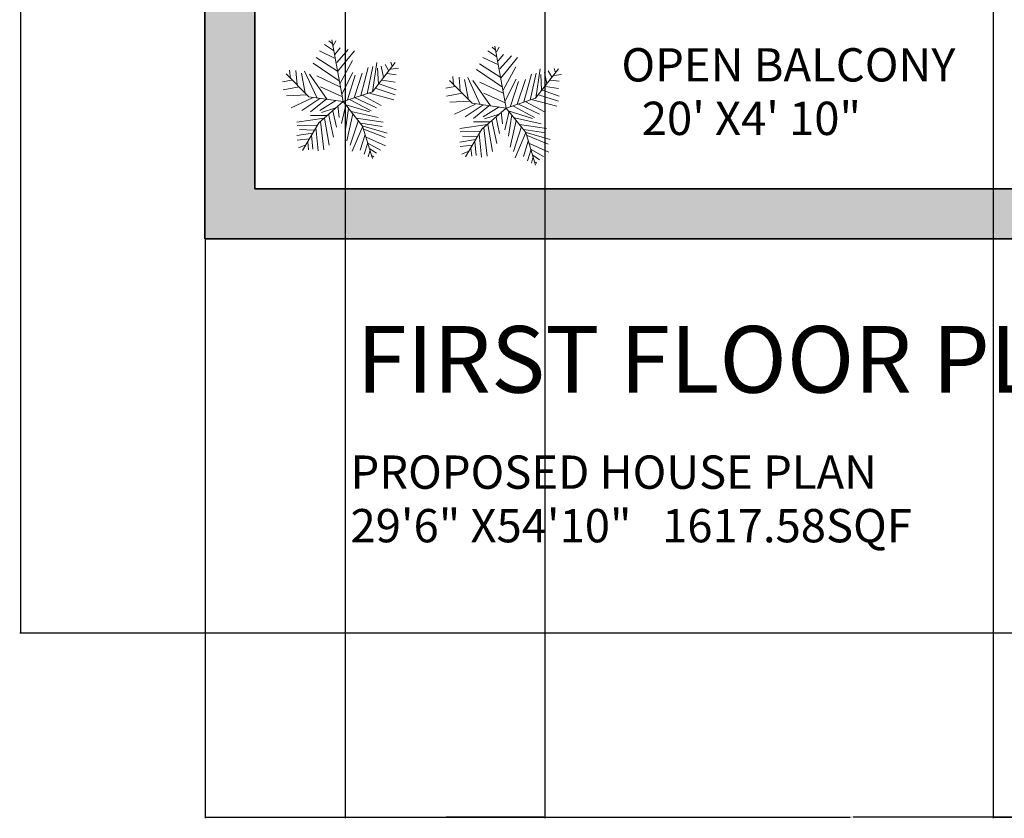
# Model space of a CAD drawing. Units: inches. Extents: x 2070 to 4408, y 1595 to 4269.
# Tile 1 of 20: x 2070 to 2247, y 1595 to 1739. Entities that reach past the tile are written whole.
import ezdxf

# ---------------------------------------------------------------- set-up
doc = ezdxf.new("R2010")
doc.units = ezdxf.units.IN
for name, color, linetype, lineweight in [('A-ANNO-DIMS', 2, 'Continuous', 18), ('A-ANNO-TITL', 7, 'Continuous', 25), ('A-AREA-IDEN', 7, 'Continuous', 18), ('A-WALL', 7, 'Continuous', 35), ('L-PLNT', 3, 'Continuous', 13)]:
    doc.layers.add(name, color=color, linetype=linetype, lineweight=lineweight)
doc.layers.add('A-WALL-PATT', color=18, linetype='Continuous', lineweight=13, true_color=0x000000)
doc.styles.get("Standard").update_dxf_attribs({"font": 'arial.ttf'})
doc.dimstyles.get("Standard").update_dxf_attribs({"dimtxt": 0.18, "dimasz": 0.18, "dimexe": 0.18, "dimexo": 0.0625, "dimgap": 0.09, "dimtad": 0, "dimtih": 1, "dimtoh": 1, "dimdec": 4, "dimzin": 0, "dimdsep": 46, "dimtxsty": 'Standard', "dimcen": 0.09, "dimadec": 0, "dimazin": 0, "dimtfac": 1, "dimtdec": 4, "dimtofl": 0, "dimtmove": 0, "dimatfit": 3, "dimfxl": 1, "dimtolj": 1, "dimtzin": 0, "dimarcsym": 0})

# ---------------------------------------------------------------- blocks, each defined once
blk = doc.blocks.new('Trees - Imperial')
for p, q in [((-10.186, 53.64), (-13.084, 55.962)), ((0, 0), (-10.5, 57)), ((-9.099, 51.782), (-6.563, 55.962)), ((-7.288, 39.707), (-21.778, 46.673)), ((-8.737, 47.138), (-17.069, 52.711)), ((-7.65, 43.423), (-2.578, 49.46)), ((-5.839, 35.992), (4.667, 48.067)), ((-5.114, 27.632), (10.463, 46.673)), ((-5.114, 28.097), (-24.676, 40.636)), ((-2.941, 16.486), (8.652, 37.85)), ((44.153, 36.456), (45.239, 32.741)), ((-48.585, 21.131), (-49.309, 29.026)), ((-43.513, 28.561), (-42.427, 15.558)), ((-35.544, 28.097), (-24.314, 3.947)), ((-3.665, 19.273), (-27.574, 35.527)), ((16.259, 5.805), (23.142, 31.348)), ((22.055, 7.198), (27.489, 32.277)), ((27, 9), (48, 36)), ((27.127, 9.056), (31.112, 35.992)), ((31.836, 30.883), (32.561, 16.486)), ((35.096, 32.741), (37.27, 22.524)), ((38.719, 34.134), (41.979, 28.561)), ((43.791, 29.954), (51.036, 30.883)), ((-47.498, 19.737), (-55.83, 18.344)), ((-31.5, 4.5), (-52.5, 25.5)), ((-38.442, 26.239), (-34.819, 7.663)), ((-14.533, 2.09), (-30.834, 25.31)), ((-24.314, 23.917), (-2.941, 13.7)), ((-1.129, 6.734), (9.014, 26.704)), ((3.942, 1.625), (11.187, 24.381)), ((10.101, 3.483), (17.708, 26.239)), ((36.183, 19.737), (48.137, 17.88)), ((40.53, 25.775), (48.862, 24.846)), ((-40.615, 13.7), (-55.105, 10.913)), ((-20.691, 13.7), (-1.129, 4.876)), ((29.662, 12.307), (48.137, 6.269)), ((33.285, 16.486), (48.862, 10.913)), ((-33.37, 6.269), (-52.207, 5.34)), ((-28.299, 3.483), (-47.86, -5.805)), ((-21.416, 3.018), (-38.079, -8.128)), ((0, 0), (-31.5, 4.5)), ((-15.982, 2.09), (-30.11, -9.521)), ((0, 0), (-22.5, -19.5)), ((-6.563, 1.161), (-21.416, -8.128)), ((0, 0), (27, 9)), ((0, 0), (18, -22.5)), ((6.478, 1.625), (26.04, -8.592)), ((11.187, 3.483), (30.749, -5.805)), ((18.07, 5.805), (35.096, -3.483)), ((24.229, 7.663), (46.688, 1.625)), ((-6.563, -5.805), (-19.967, -9.985)), ((-9.461, -8.592), (-6.201, -23.453)), ((-4.752, -3.483), (-3.665, -14.629)), ((2.493, -3.019), (-1.491, -20.202)), ((1.769, -2.555), (24.229, -9.521)), ((5.029, -6.27), (2.131, -25.775)), ((7.565, -9.056), (32.198, -14.629)), ((-17.431, -15.094), (-42.789, -18.809)), ((-15.257, -12.772), (-30.11, -12.772)), ((-17.069, -15.094), (-12.721, -40.172)), ((-13.446, -11.378), (-8.737, -32.741)), ((9.014, -11.378), (3.58, -35.992)), ((14.085, -16.951), (6.478, -40.172)), ((12.274, -15.094), (36.907, -18.809)), ((-24.314, -21.596), (-42.427, -22.06)), ((-26.849, -26.24), (-40.253, -25.775)), ((-22.5, -19.5), (-37.5, -45)), ((-25.038, -23.918), (-22.865, -45.281)), ((-20.691, -18.345), (-17.793, -44.352)), ((18.07, -22.524), (8.289, -45.745)), ((16.259, -19.738), (36.183, -22.989)), ((18, -22.5), (27, -52.5)), ((18.433, -22.524), (40.53, -29.026)), ((19.157, -25.311), (38.719, -33.206)), ((-28.299, -29.026), (-42.789, -31.348)), ((-30.834, -34.135), (-42.427, -35.528)), ((-29.023, -30.884), (-27.936, -43.887)), ((20.244, -30.419), (15.897, -44.816)), ((21.331, -32.741), (39.081, -40.636)), ((-34.457, -39.708), (-40.978, -42.494)), ((-32.646, -36.921), (-31.921, -44.352)), ((22.78, -37.85), (19.519, -48.532)), ((22.78, -38.314), (34.372, -44.816)), ((24.591, -43.423), (30.749, -47.603)), ((24.591, -45.745), (23.142, -50.854)), ((26.764, -49.925), (28.213, -50.854))]:
    blk.add_line(p, q)
blk = doc.blocks.new('*D24')
at = {"layer": 'A-ANNO-DIMS', "color": 0, "lineweight": -2, "transparency": 16777216}
for p, q in [((2103.13, 2291.4), (2069.84, 2291.4)), ((2070.02, 2291.22), (2070.02, 1960.08)), ((2070.02, 1628.58), (2070.02, 1959.72)), ((2336.13, 1628.4), (2069.84, 1628.4))]:
    blk.add_line(p, q, dxfattribs=at)
at = {"layer": 'A-ANNO-DIMS', "color": 0, "transparency": 16777216}
for points in [[(2069.99, 2291.22), (2070.05, 2291.22), (2070.02, 2291.4)], [(2069.99, 1628.58), (2070.05, 1628.58), (2070.02, 1628.4)]]:
    blk.add_solid(points, dxfattribs=at)
at = {"layer": 'Defpoints', "color": 0, "transparency": 16777216}
for p in [(2070.02, 2291.4), (2103.2, 2291.4), (2336.2, 1628.4)]:
    blk.add_point(p, dxfattribs=at)
at = {"layer": 'A-ANNO-DIMS', "color": 0, "transparency": 16777216, "insert": (2070.02, 1959.9), "char_height": 0.18, "attachment_point": 5}
blk.add_mtext('\\A1;663', dxfattribs=at)
blk = doc.blocks.new('*D25')
at = {"layer": 'A-ANNO-DIMS', "color": 0, "lineweight": -2, "transparency": 16777216}
for p, q in [((2103.2, 1699.34), (2103.2, 1595.04)), ((2336.2, 1699.34), (2336.2, 1595.04)), ((2103.38, 1595.22), (2219.41, 1595.22)), ((2336.02, 1595.22), (2219.99, 1595.22))]:
    blk.add_line(p, q, dxfattribs=at)
at = {"layer": 'A-ANNO-DIMS', "color": 0, "transparency": 16777216}
for points in [[(2103.38, 1595.25), (2103.38, 1595.19), (2103.2, 1595.22)], [(2336.02, 1595.25), (2336.02, 1595.19), (2336.2, 1595.22)]]:
    blk.add_solid(points, dxfattribs=at)
at = {"layer": 'Defpoints', "color": 0, "transparency": 16777216}
for p in [(2103.2, 1699.4), (2336.2, 1699.4), (2336.2, 1595.22)]:
    blk.add_point(p, dxfattribs=at)
at = {"layer": 'A-ANNO-DIMS', "color": 0, "transparency": 16777216, "insert": (2219.7, 1595.22), "char_height": 0.18, "attachment_point": 5}
blk.add_mtext('\\A1;233', dxfattribs=at)
blk = doc.blocks.new('*D29')
at = {"layer": 'A-ANNO-DIMS', "color": 0, "lineweight": -2, "transparency": 16777216}
for p, q in [((2128.44, 2150.34), (2128.44, 1595.04)), ((2164.44, 2150.34), (2164.44, 1595.04)), ((2128.62, 1595.22), (2146.22, 1595.22)), ((2164.26, 1595.22), (2146.65, 1595.22))]:
    blk.add_line(p, q, dxfattribs=at)
at = {"layer": 'A-ANNO-DIMS', "color": 0, "transparency": 16777216}
for points in [[(2128.62, 1595.25), (2128.62, 1595.19), (2128.44, 1595.22)], [(2164.26, 1595.25), (2164.26, 1595.19), (2164.44, 1595.22)]]:
    blk.add_solid(points, dxfattribs=at)
at = {"layer": 'Defpoints', "color": 0, "transparency": 16777216}
for p in [(2128.44, 2150.4), (2164.44, 2150.4), (2164.44, 1595.22)]:
    blk.add_point(p, dxfattribs=at)
at = {"layer": 'A-ANNO-DIMS', "color": 0, "transparency": 16777216, "insert": (2146.44, 1595.22), "char_height": 0.18, "attachment_point": 5}
blk.add_mtext('\\A1;36', dxfattribs=at)
blk = doc.blocks.new('*D32')
at = {"layer": 'A-ANNO-DIMS', "color": 0, "lineweight": -2, "transparency": 16777216}
for p, q in [((2245.2, 2230.58), (2245.2, 1595.04)), ((2340.2, 2230.58), (2340.2, 1595.04)), ((2245.38, 1595.22), (2292.48, 1595.22)), ((2340.02, 1595.22), (2292.92, 1595.22))]:
    blk.add_line(p, q, dxfattribs=at)
at = {"layer": 'A-ANNO-DIMS', "color": 0, "transparency": 16777216}
for points in [[(2245.38, 1595.25), (2245.38, 1595.19), (2245.2, 1595.22)], [(2340.02, 1595.25), (2340.02, 1595.19), (2340.2, 1595.22)]]:
    blk.add_solid(points, dxfattribs=at)
at = {"layer": 'Defpoints', "color": 0, "transparency": 16777216}
for p in [(2245.2, 2230.65), (2340.2, 2230.65), (2340.2, 1595.22)]:
    blk.add_point(p, dxfattribs=at)
at = {"layer": 'A-ANNO-DIMS', "color": 0, "transparency": 16777216, "insert": (2292.7, 1595.22), "char_height": 0.18, "attachment_point": 5}
blk.add_mtext('\\A1;95', dxfattribs=at)

msp = doc.modelspace()

# ---------------------------------------------------------------- hatches: boundary and pattern name
at = {"layer": 'A-WALL-PATT'}
h = msp.add_hatch(color=256, dxfattribs=at)
h.dxf.hatch_style = 1
h.paths.add_polyline_path([(2346.196, 2218.3995), (2346.196, 2282.3995), (2340.196, 2282.3995), (2340.196, 2212.3995), (2345.5866, 2212.3995), (2346.196, 2212.3995)], flags=0)
h.paths.add_polyline_path([(2245.196, 2282.3995), (2239.196, 2282.3995), (2239.196, 2186.3995), (2244.5866, 2186.3995), (2245.196, 2186.3995)], flags=0)
h.paths.add_polyline_path([(2340.196, 2230.6455), (2245.196, 2230.6455), (2245.196, 2224.6455), (2340.196, 2224.6455)], flags=0)
h.paths.add_polyline_path([(2245.196, 2150.3995), (2239.196, 2150.3995), (2164.4362, 2150.3995), (2164.4362, 2144.3995), (2239.196, 2144.3995), (2239.196, 2086.3995), (2239.196, 2067.2711), (2244.5866, 2067.2711), (2245.196, 2067.2711), (2245.196, 2144.3995)], flags=0)
h.paths.add_polyline_path([(2346.196, 2176.3995), (2340.196, 2176.3995), (2340.196, 2086.3995), (2346.196, 2086.3995), (2346.196, 2125.318)], flags=0)
h.paths.add_polyline_path([(2446.196, 2086.3995), (2346.196, 2086.3995), (2340.196, 2086.3995), (2340.196, 2080.3995), (2446.196, 2080.3995)], flags=0)
h.paths.add_polyline_path([(2455.196, 2291.3995), (2103.196, 2291.3995), (2103.196, 1699.3995), (2336.196, 1699.3995), (2336.196, 1628.3995), (2345.196, 1628.3995), (2446.196, 1628.3995), (2454.8846, 1628.3995), (2454.8846, 1699.3995)])
h.paths.add_polyline_path([(2446.196, 2282.3995), (2446.196, 2218.3995), (2446.196, 2212.3995), (2446.196, 2086.3995), (2446.196, 2080.3995), (2446.196, 1708.3995), (2446.196, 1637.3995), (2345.196, 1637.3995), (2345.196, 1699.3995), (2345.196, 1708.3995), (2336.196, 1708.3995), (2112.196, 1708.3995), (2112.196, 2282.3995), (2239.196, 2282.3995), (2245.196, 2282.3995), (2356.196, 2282.3995)], flags=16)
h.paths.add_polyline_path([(2245.196, 2150.3995), (2245.196, 2144.3995), (2245.196, 2067.2711), (2244.5866, 2067.2711), (2239.196, 2067.2711), (2239.196, 2065.6988), (2203.2929, 2065.6988, 0.40145271), (2239.196, 2031.3337), (2244.5866, 2031.3337), (2245.196, 2031.2711), (2245.196, 1924.1525), (2239.196, 1924.1525), (2239.196, 1922.5803), (2203.2929, 1922.5803, 0.40145271), (2239.196, 1888.2151), (2244.5866, 1888.2151), (2245.196, 1888.1525), (2245.196, 1748.3995), (2339.196, 1748.4621, -0.40145271), (2303.2929, 1782.8272), (2303.2585, 1782.8272), (2303.2585, 1784.3995), (2339.196, 1784.3995), (2339.196, 1877.2067), (2291.196, 1877.2067), (2291.196, 1883.2067), (2291.196, 1946.3995), (2291.196, 1952.3995), (2291.196, 2086.3995), (2297.196, 2086.3995), (2302.196, 2086.3995), (2302.196, 2081.0259), (2303.7633, 2081.0259), (2303.7633, 2080.3995), (2338.0148, 2080.3995, 0.00437129), (2338.0203, 2081.0259), (2338.0203, 2086.3995), (2340.196, 2086.3995), (2340.196, 2176.4621), (2345.5866, 2176.4621, 0.40145271), (2381.4896, 2210.8272), (2345.5866, 2210.8272), (2345.5866, 2212.3995), (2340.196, 2212.3995), (2340.196, 2224.6455), (2245.196, 2224.6455), (2245.196, 2186.3995), (2244.5866, 2186.3995), (2239.196, 2186.3995), (2239.196, 2184.8272), (2203.2929, 2184.8272, 0.40145271), (2239.196, 2150.4621), (2244.5866, 2150.4621)], flags=0)
h.paths.add_polyline_path([(2346.196, 2282.3995), (2346.196, 2218.3995), (2377.1813, 2218.3995), (2377.1813, 2212.3995), (2346.196, 2212.3995), (2345.5866, 2212.3995), (2340.196, 2212.3995), (2340.196, 2224.6455), (2245.196, 2224.6455), (2245.196, 2230.6455), (2245.196, 2282.3995), (2292.696, 2256.5225), (2340.196, 2282.3995)], flags=0)
h.paths.add_polyline_path([(2346.196, 2086.3995), (2340.196, 2086.3995), (2340.196, 2080.3995), (2446.196, 2080.3995), (2431.196, 2016.3995), (2446.196, 1952.3995), (2412.196, 1952.3995), (2412.196, 2080.3995), (2340.196, 2080.3995), (2340.196, 2086.3995), (2340.196, 2176.3995), (2346.196, 2176.3995), (2346.196, 2125.318)], flags=0)
h.paths.add_polyline_path([(2186.508, 2270.0471, -0.03755288), (2186.9712, 2269.8581), (2186.9164, 2270.112, -0.02759121)], flags=0)
h.paths.add_polyline_path([(2183.955, 2273.7766, 1), (2188.2945, 2273.7766, 1)], flags=0)
h.paths.add_polyline_path([(2142.5261, 2274.6158, -0.03707541), (2142.5672, 2275.1696), (2142.5672, 2276.826), (2119.8759, 2276.826), (2119.8759, 2263.0962), (2140.4332, 2263.0962), (2142.5672, 2263.0962), (2142.5672, 2274.0621, -0.03707541)], flags=0)
h.paths.add_polyline_path([(2209.8974, 2263.0962), (2209.8974, 2262.2079), (2190.8042, 2262.2079), (2190.8042, 2263.0962)], flags=0)
h.paths.add_polyline_path([(2210.6382, 2276.1833), (2210.6382, 2263.9844), (2190.2185, 2263.9844), (2190.2185, 2276.1833)], flags=0)
h.paths.add_polyline_path([(2188.4362, 2273.7766, -1), (2183.8133, 2273.7766, -1)], flags=0)
h.paths.add_polyline_path([(2245.196, 2150.3995), (2245.196, 2144.3995), (2245.196, 2067.2711), (2239.196, 2067.2711), (2239.196, 2080.3995), (2172.196, 2080.3995), (2172.196, 2000.3995), (2239.196, 2000.3995), (2239.196, 1940.3995), (2159.0187, 1940.3995), (2123.0187, 1940.3995), (2112.196, 1940.3995), (2112.196, 1946.3995), (2123.0187, 1946.3995), (2123.0187, 1982.2238), (2124.586, 1982.2238), (2124.586, 1982.1895, -0.40145271), (2158.8429, 1946.3995), (2159.0187, 1946.3995), (2239.196, 1946.3995), (2239.196, 1994.3995), (2112.196, 1994.3995), (2112.196, 2000.3995), (2139.196, 2040.3995), (2112.196, 2080.3995), (2112.196, 2086.3995), (2239.196, 2086.3995), (2239.196, 2144.3995), (2209.5809, 2144.3995), (2209.5809, 2136.3995), (2203.0809, 2136.3995), (2205.0809, 2130.3996, -0.70257121), (2199.081, 2116.3995, -0.70256205), (2193.0809, 2130.3994), (2195.0809, 2136.3995), (2192.0809, 2136.3995), (2192.0809, 2134.8995), (2189.0809, 2134.8995), (2189.0809, 2135.8995), (2191.0809, 2135.8995), (2191.0809, 2136.3995), (2188.5809, 2136.3995), (2188.5809, 2144.3995), (2164.2481, 2144.3995, -0.39385849), (2130.0035, 2109.5491), (2130.0035, 2109.5147), (2128.4362, 2109.5147), (2128.4362, 2144.3995), (2112.196, 2144.3995), (2112.196, 2150.3995), (2128.4362, 2150.3995), (2128.4362, 2150.7127), (2164.4362, 2150.7127), (2164.4362, 2150.3995), (2239.196, 2150.3995)], flags=0)
h.paths.add_polyline_path([(2188.2075, 2266.8735), (2188.2075, 2211.8632, -0.41421356), (2185.4833, 2209.1391), (2146.7995, 2209.1391, -0.41421356), (2144.0754, 2211.8632), (2144.0754, 2266.8735, -0.41421356), (2146.7995, 2269.5976), (2185.4833, 2269.5976, -0.41421356)], flags=0)
h.paths.add_polyline_path([(2185.0844, 2273.7766, -1), (2187.1651, 2273.7766, -1)], flags=0)
h.paths.add_polyline_path([(2182.0486, 2259.2932), (2168.0953, 2259.2932), (2168.0953, 2260.8424), (2163.7261, 2260.8424), (2163.7261, 2259.2932), (2149.7727, 2259.2932), (2149.7727, 2266.3352), (2163.7261, 2266.3352), (2163.7261, 2261.9839), (2168.0953, 2261.9839), (2168.0953, 2266.3352), (2182.0486, 2266.3352)], flags=0)
h.paths.add_polyline_path([(2148.2585, 2250.2051), (2153.0615, 2241.8861, 0.39807048)], flags=0)
h.paths.add_polyline_path([(2162.7572, 2247.2885), (2153.1461, 2241.7396), (2148.1083, 2250.4653), (2157.7194, 2256.0142)], flags=0)
h.paths.add_polyline_path([(2162.6726, 2247.4351, -0.39286196), (2157.8415, 2255.6313), (2157.6431, 2255.6313), (2157.8696, 2255.7541)], flags=0)
h.paths.add_polyline_path([(2164.2604, 2145.339), (2164.4362, 2144.3995), (2164.4362, 2150.3995), (2164.2604, 2150.7127)], flags=0)
h.paths.add_polyline_path([(2208.5809, 2142.6495), (2208.5809, 2138.3995, -0.41421356), (2207.8309, 2137.3995), (2190.5809, 2137.3995, -0.41421356), (2189.5809, 2138.1495), (2189.5809, 2142.3995, -0.41421356), (2190.3309, 2143.3995), (2207.5809, 2143.3995, -0.41421356)], flags=0)
h.paths.add_polyline_path([(2147.957, 2229.9119), (2154.7494, 2223.1195, 0.39807048)], flags=0)
h.paths.add_polyline_path([(2162.7165, 2230.8473), (2154.8691, 2222.9998), (2147.7446, 2230.1244), (2155.592, 2237.9718)], flags=0)
h.paths.add_polyline_path([(2162.5969, 2230.9669, -0.39807048), (2155.8044, 2237.7594)], flags=0)
h.paths.add_polyline_path([(2391.8776, 2049.9192), (2408.5766, 2049.9192), (2408.5766, 2033.2202), (2408.5766, 1983.123), (2408.5766, 1966.4239), (2391.8776, 1966.4239), (2391.8776, 1983.123), (2341.7804, 1983.123), (2341.7804, 2033.2202), (2391.8776, 2033.2202)], flags=0)
h.paths.add_polyline_path([(2144.1055, 2274.6158, 1), (2148.445, 2274.6158, 1)], flags=0)
h.paths.add_polyline_path([(2148.5867, 2274.6158, -1), (2143.9638, 2274.6158, -1)], flags=0)
h.paths.add_polyline_path([(2145.2349, 2274.6158, -1), (2147.3156, 2274.6158, -1)], flags=0)
edge = h.paths.add_edge_path(flags=0)
edge.add_ellipse((2400.5951, 2040.9436), major_axis=(-4.5109, 0), ratio=0.97544784, start_angle=180, end_angle=270, ccw=False)
edge.add_ellipse((2400.5951, 2040.9436), major_axis=(-4.5109, 0), ratio=0.97544784, start_angle=90, end_angle=180, ccw=False)
edge.add_ellipse((2400.5951, 2040.9436), major_axis=(-4.5109, 0), ratio=0.97544784, start_angle=0, end_angle=90, ccw=False)
edge.add_ellipse((2400.5951, 2040.9436), major_axis=(-4.5109, 0), ratio=0.97544784, start_angle=270, end_angle=360, ccw=False)
h.paths.add_polyline_path([(2199.0809, 2117.3995, -0.73452973), (2195.0809, 2130.3995), (2203.081, 2130.3995, -0.73453329)], flags=0)
h.paths.add_polyline_path([(2141.9147, 2276.0353), (2141.9147, 2263.9844), (2120.4685, 2263.9844), (2120.4685, 2276.0353)], flags=0)
h.paths.add_polyline_path([(2138.4481, 2273.4072), (2138.4481, 2266.7226), (2133.2801, 2266.7226), (2133.2801, 2273.4072)], flags=0)
h.paths.add_polyline_path([(2137.9691, 2272.9175), (2137.9691, 2272.204), (2135.4229, 2272.204), (2135.4229, 2271.6329), (2135.3221, 2270.1051), (2135.3221, 2269.0265), (2135.4229, 2268.6811), (2135.4229, 2267.2011), (2133.7212, 2267.2011), (2133.7212, 2268.6811), (2133.7983, 2269.9587), (2133.7983, 2271.2758), (2133.7212, 2271.6329), (2133.7212, 2273.0065), (2135.717, 2273.0065), (2135.717, 2272.9175)], flags=0)
h.paths.add_polyline_path([(2137.9215, 2271.8264), (2137.9215, 2271.3786), (2137.5182, 2271.3786), (2136.9355, 2271.3786), (2136.3529, 2271.3786), (2135.7703, 2271.3786), (2135.7703, 2271.8264), (2136.1736, 2271.8264), (2136.7562, 2271.8264), (2137.3389, 2271.8264)], flags=0)
h.paths.add_polyline_path([(2137.9215, 2271.692), (2137.5182, 2271.692), (2136.9355, 2271.513), (2137.3389, 2271.513)], flags=0)
h.paths.add_polyline_path([(2136.3529, 2271.692), (2135.7703, 2271.513), (2136.1736, 2271.513), (2136.7562, 2271.692)], flags=0)
h.paths.add_polyline_path([(2137.9215, 2271.513), (2137.5182, 2271.513), (2136.7562, 2271.747), (2136.7562, 2271.692), (2137.3389, 2271.692)], flags=0)
h.paths.add_polyline_path([(2137.8207, 2270.4664), (2137.8207, 2270.0971), (2137.8207, 2269.627), (2137.8207, 2269.1569), (2137.8207, 2268.6868), (2137.3837, 2268.6868), (2136.6442, 2268.6868), (2135.9271, 2268.6868), (2135.9271, 2269.0562), (2135.9271, 2269.5263), (2135.9271, 2269.9963), (2135.9271, 2270.4664), (2136.3641, 2270.4664), (2137.0812, 2270.4664)], flags=0)
h.paths.add_polyline_path([(2137.3837, 2269.627), (2137.8207, 2269.627), (2137.8207, 2269.5263), (2137.3837, 2269.5263), (2137.3837, 2269.1569), (2137.8207, 2269.1569), (2137.3837, 2269.0562), (2137.3837, 2268.6868), (2137.0812, 2268.6868), (2137.0812, 2269.0562), (2136.6442, 2269.0562), (2136.6442, 2268.6868), (2136.3641, 2268.6868), (2136.3641, 2269.0562), (2135.9271, 2269.0562), (2135.9271, 2269.1569), (2136.3641, 2269.1569), (2136.3641, 2269.5263), (2135.9271, 2269.5263), (2135.9271, 2269.627), (2136.3641, 2269.627), (2136.3641, 2269.9963), (2135.9271, 2269.9963), (2136.3641, 2270.0971), (2136.3641, 2270.4664), (2136.6442, 2270.4664), (2136.6442, 2270.0971), (2137.0812, 2270.0971), (2137.0812, 2270.4664), (2137.3837, 2270.4664), (2137.3837, 2270.0971), (2137.8207, 2270.0971), (2137.3837, 2269.9963)], flags=0)
h.paths.add_polyline_path([(2137.5182, 2271.8264), (2137.5182, 2271.692), (2137.3389, 2271.3786), (2137.3389, 2271.513)], flags=0)
h.paths.add_polyline_path([(2137.8179, 2267.8138), (2137.8179, 2267.6879), (2137.1876, 2267.6879), (2136.4733, 2267.6879), (2135.759, 2267.6879), (2135.759, 2267.8138), (2136.3893, 2267.8138), (2137.1036, 2267.8138)], flags=0)
h.paths.add_polyline_path([(2137.0812, 2269.9963), (2137.0812, 2269.627), (2137.0812, 2269.1569), (2136.6442, 2269.1569), (2136.6442, 2269.5263), (2136.6442, 2269.9963)], flags=0)
h.paths.add_polyline_path([(2136.3529, 2271.8264), (2136.3529, 2271.692), (2136.1736, 2271.3786), (2136.1736, 2271.513)], flags=0)
h.paths.add_polyline_path([(2136.4733, 2267.8138), (2136.4733, 2267.6879), (2136.3893, 2267.6879), (2136.3893, 2267.8138)], flags=0)
h.paths.add_polyline_path([(2407.9087, 2032.5522), (2407.9087, 1983.7909), (2359.81, 1983.7909, -0.00912788), (2359.0575, 1983.7909), (2342.4483, 1983.7909), (2342.4483, 2032.5522)], flags=0)
h.paths.add_polyline_path([(2389.1838, 2023.1358), (2353.7856, 2023.1358), (2353.7856, 1985.4867, -0.09210376), (2350.2788, 1988.655), (2350.2788, 2026.6426), (2389.1838, 2026.6426)], flags=0)
h.paths.add_polyline_path([(2352.6166, 2024.3048), (2351.4477, 2024.3048), (2351.4477, 2025.4737), (2352.6166, 2025.4737)], flags=0)
h.paths.add_polyline_path([(2399.6319, 2026.7589), (2404.3661, 2026.7589, -0.41421356), (2407.0379, 2024.087), (2407.0379, 2013.4908, -0.41421356), (2404.3661, 2010.819), (2399.6319, 2010.819, -0.41421356), (2396.96, 2013.4908), (2396.96, 2024.087, -0.41421356)], flags=0)
h.paths.add_polyline_path([(2399.6319, 2026.0909), (2404.3661, 2026.0909, -0.41421356), (2406.37, 2024.087), (2406.37, 2013.4908, -0.41421356), (2404.3661, 2011.487), (2399.6319, 2011.487, -0.41421356), (2397.628, 2013.4908), (2397.628, 2024.087, -0.41421356)], flags=0)
h.paths.add_polyline_path([(2399.6319, 2002.3217), (2404.3661, 2002.3217, -0.41421356), (2407.0379, 1999.6498), (2407.0379, 1989.0536, -0.41421356), (2404.3661, 1986.3818), (2399.6319, 1986.3818, -0.41421356), (2396.96, 1989.0536), (2396.96, 1999.6498, -0.41421356)], flags=0)
h.paths.add_polyline_path([(2399.6319, 2001.6537), (2404.3661, 2001.6537, -0.41421356), (2406.37, 1999.6498), (2406.37, 1989.0536, -0.41421356), (2404.3661, 1987.0497), (2399.6319, 1987.0497, -0.41421356), (2397.628, 1989.0536), (2397.628, 1999.6498, -0.41421356)], flags=0)
edge = h.paths.add_edge_path(flags=0)
edge.add_ellipse((2400.5951, 1975.3996), major_axis=(-4.5109, 0), ratio=0.97544784, start_angle=-180, end_angle=-90, ccw=False)
edge.add_ellipse((2400.5951, 1975.3996), major_axis=(-4.5109, 0), ratio=0.97544784, start_angle=90, end_angle=180, ccw=False)
edge.add_ellipse((2400.5951, 1975.3996), major_axis=(-4.5109, 0), ratio=0.97544784, start_angle=0, end_angle=90, ccw=False)
edge.add_ellipse((2400.5951, 1975.3996), major_axis=(-4.5109, 0), ratio=0.97544784, start_angle=-90, end_angle=0, ccw=False)
h.paths.add_polyline_path([(2345.196, 1910.3995), (2366.4386, 1910.3995), (2366.4386, 1925.4555), (2392.3856, 1925.4555), (2392.3856, 1933.5025), (2400.1399, 1925.4555), (2392.3856, 1919.8795), (2392.3856, 1925.4555), (2366.4386, 1925.4555), (2366.4386, 1910.3995), (2381.196, 1910.3995), (2405.196, 1910.3995), (2405.196, 1898.3995), (2446.196, 1898.3995), (2446.196, 1886.3995), (2405.196, 1886.3995), (2405.196, 1874.3995), (2446.196, 1874.3995), (2446.196, 1862.3995), (2405.196, 1862.3995), (2405.196, 1850.3995), (2446.196, 1850.3995), (2446.196, 1838.3995), (2405.196, 1838.3995), (2405.196, 1826.3995), (2446.196, 1826.3995), (2446.196, 1814.3995), (2405.196, 1814.3995), (2405.196, 1802.3995), (2446.196, 1802.3995), (2446.196, 1798.3995), (2446.196, 1792.3995), (2405.196, 1792.3995), (2405.196, 1910.3995), (2381.196, 1910.3995), (2381.196, 1792.3995), (2345.196, 1792.3995)], flags=0)
h.paths.add_polyline_path([(2333.0944, 1863.3993, -0.41421356), (2334.7225, 1861.7712), (2334.7225, 1859.329), (2335.2653, 1859.329, -0.41421356), (2337.4361, 1857.1582), (2337.4361, 1843.862, -0.41421356), (2335.2653, 1841.6911, -0.41421356), (2337.4361, 1839.5203), (2337.4361, 1827.5808, -0.41421356), (2335.2653, 1825.41, -0.41421356), (2337.4361, 1823.2392), (2337.4361, 1808.5862, -0.41421356), (2335.2653, 1806.4153), (2334.7225, 1806.4153), (2334.7225, 1803.9732, -0.41421356), (2333.0944, 1802.3451), (2317.356, 1802.3451), (2317.0846, 1802.3451, -0.41421356), (2315.7279, 1803.7018), (2315.7279, 1803.8646), (2313.8284, 1803.8646, -0.41421356), (2311.6576, 1806.0354), (2311.6576, 1823.2015, -0.39597602), (2313.6834, 1825.3765, -0.43384798), (2311.6576, 1827.2718), (2311.6576, 1839.761, -0.41421356), (2313.5571, 1841.6604), (2313.8284, 1841.6604), (2333.8159, 1841.6604, -0.04213623), (2334.1798, 1841.6911, -0.41421356), (2332.009, 1843.862), (2332.009, 1857.1582, -0.41421356), (2334.1798, 1859.329), (2317.356, 1859.329), (2317.0846, 1859.329, -0.41421356), (2315.7279, 1860.6858), (2315.7279, 1862.0426, -0.41421356), (2317.0846, 1863.3993), (2317.356, 1863.3993)], flags=0)
h.paths.add_polyline_path([(2208.8475, 1848.9818), (2208.8475, 1840.9741, -0.41421356), (2207.0458, 1839.1724), (2206.5453, 1839.1721), (2206.5453, 1838.7218, -0.40985861), (2204.7704, 1836.9203), (2183.7501, 1836.9203, -0.41858196), (2181.9216, 1838.7218), (2181.9216, 1839.1721), (2181.421, 1839.1724, -0.41421356), (2179.6193, 1840.9741), (2179.6193, 1848.6817, -0.44064415), (2185.1126, 1854.9874), (2203.3852, 1854.9874, -0.45707961)], flags=0)
h.paths.add_polyline_path([(2204.243, 1848.4815), (2204.243, 1848.4815, 0.41725335), (2202.2204, 1850.4833), (2186.2049, 1850.4833, 0.4111805), (2184.2237, 1848.4815), (2184.2237, 1848.4815, -0.4111807), (2186.2049, 1850.4833), (2202.2204, 1850.4833, -0.41725315)], flags=0)
h.paths.add_polyline_path([(2234.7177, 1830.228), (2234.7176, 1781.6047, -0.41421356), (2233.4381, 1780.3252), (2218.6064, 1780.3252, -0.41421356), (2217.8387, 1781.0929), (2217.8387, 1783.3961, -0.41421356), (2218.6064, 1784.1639), (2218.6065, 1796.9595, -0.41421356), (2219.886, 1798.239, -0.41421356), (2218.6065, 1799.5186), (2218.6065, 1812.3142, -0.41421356), (2219.8861, 1813.5938, -0.41421356), (2218.6065, 1814.8733), (2218.6065, 1827.6689, -0.41421356), (2217.8388, 1828.4367), (2217.8388, 1830.7399, -0.41421356), (2218.6065, 1831.5076), (2233.4382, 1831.5076, -0.41421356)], flags=0)
h.paths.add_polyline_path([(2230.6344, 1827.6689, -0.41421356), (2231.4021, 1826.9012), (2231.4021, 1784.9316, -0.41421356), (2230.6343, 1784.1639), (2221.1853, 1784.1639), (2221.1853, 1827.6689)], flags=0)
h.paths.add_polyline_path([(2222.7208, 1798.239), (2221.6971, 1798.239), (2221.6971, 1813.5938), (2222.7208, 1813.5938)], flags=0)
h.paths.add_polyline_path([(2206.5453, 1773.935), (2206.5453, 1773.4848), (2206.9457, 1773.4848), (2207.0458, 1773.4845, -0.41421356), (2208.8475, 1771.6827), (2208.8475, 1763.675, -0.44222432), (2203.6505, 1757.6695), (2185.3851, 1757.6695, -0.45508402), (2179.6193, 1763.9752), (2179.6193, 1771.6827, -0.41421356), (2181.421, 1773.4845), (2181.421, 1773.4848), (2181.9216, 1773.4848), (2181.9216, 1773.935, -0.40985861), (2183.6965, 1775.7366), (2204.7167, 1775.7366, -0.41858196)], flags=0)
h.paths.add_polyline_path([(2202.2619, 1762.1736), (2186.2464, 1762.1736, -0.41725315), (2184.2237, 1764.1754), (2184.2237, 1764.1754, 0.41725335), (2186.2464, 1762.1736), (2202.2619, 1762.1736, 0.4111805), (2204.243, 1764.1754), (2204.243, 1764.1754, -0.4111807)], flags=0)
h.paths.add_polyline_path([(2313.0034, 1713.1906), (2312.997, 1713.1697), (2313.0123, 1713.1612)], flags=0)
h.paths.add_polyline_path([(2305.7314, 1721.0488), (2305.6257, 1721.1994), (2305.4853, 1721.084)], flags=0)
h.paths.add_polyline_path([(2307.5562, 1726.1427), (2307.6186, 1726.1026), (2307.5737, 1726.0477), (2308.5692, 1720.6434), (2310.5345, 1721.2985), (2310.5721, 1721.411), (2310.6958, 1721.3523), (2313.8453, 1722.4021), (2314.9351, 1723.8033), (2314.9294, 1723.9165), (2315.0028, 1723.8903), (2313.874, 1722.4389), (2313.8697, 1722.4102), (2308.5692, 1720.6434), (2308.9864, 1720.122), (2309.0665, 1720.0971), (2309.053, 1720.0387), (2310.9235, 1717.7005), (2311.4182, 1717.6259), (2311.2918, 1717.2402), (2312.0655, 1716.2731), (2312.1081, 1716.2606), (2312.0969, 1716.2339), (2308.5692, 1720.6434), (2305.2249, 1717.745), (2305.232, 1717.704), (2305.1665, 1717.6944), (2308.5692, 1720.6434)], flags=0)
h.paths.add_polyline_path([(2288.2072, 1714.3431), (2288.2008, 1714.3222), (2288.216, 1714.3137)], flags=0)
h.paths.add_polyline_path([(2280.9352, 1722.2013), (2280.8295, 1722.3519), (2280.689, 1722.2365)], flags=0)
h.paths.add_polyline_path([(2282.76, 1727.2952), (2282.8224, 1727.2551), (2282.7775, 1727.2002), (2283.773, 1721.7959), (2285.7383, 1722.451), (2285.7759, 1722.5635), (2285.8995, 1722.5048), (2289.0491, 1723.5546), (2290.1389, 1724.9558), (2290.1332, 1725.069), (2290.2065, 1725.0428), (2289.0777, 1723.5915), (2289.0735, 1723.5628), (2283.773, 1721.7959), (2284.1901, 1721.2745), (2284.2703, 1721.2496), (2284.2567, 1721.1913), (2286.1273, 1718.8531), (2286.622, 1718.7785), (2286.4956, 1718.3927), (2287.2692, 1717.4256), (2287.3119, 1717.4131), (2287.3006, 1717.3864), (2283.773, 1721.7959), (2280.4286, 1718.8975), (2280.4357, 1718.8565), (2280.3703, 1718.8469), (2283.773, 1721.7959)], flags=0)
h.paths.add_polyline_path([(2302.0672, 1721.8694), (2301.8205, 1721.8572), (2301.7578, 1722.1787), (2299.415, 1724.5215), (2299.103, 1724.4694), (2299.0662, 1724.8703)], flags=0)
h.paths.add_polyline_path([(2264.5643, 1715.4956), (2264.5579, 1715.4747), (2264.5731, 1715.4662)], flags=0)
h.paths.add_polyline_path([(2257.2923, 1723.3538), (2257.1865, 1723.5044), (2257.0461, 1723.389)], flags=0)
h.paths.add_polyline_path([(2259.117, 1728.4477), (2259.1795, 1728.4077), (2259.1345, 1728.3527), (2260.13, 1722.9484), (2262.0954, 1723.6036), (2262.133, 1723.716), (2262.2566, 1723.6573), (2265.4061, 1724.7071), (2266.4959, 1726.1083), (2266.4902, 1726.2215), (2266.5636, 1726.1953), (2265.4348, 1724.744), (2265.4305, 1724.7153), (2260.13, 1722.9484), (2260.5472, 1722.427), (2260.6273, 1722.4022), (2260.6138, 1722.3438), (2262.4843, 1720.0056), (2262.979, 1719.931), (2262.8526, 1719.5452), (2263.6263, 1718.5781), (2263.6689, 1718.5656), (2263.6577, 1718.5389), (2260.13, 1722.9484), (2256.7857, 1720.05), (2256.7928, 1720.009), (2256.7273, 1719.9994), (2260.13, 1722.9484)], flags=0)
h.paths.add_polyline_path([(2277.2709, 1723.0219), (2277.0243, 1723.0097), (2276.9616, 1723.3312), (2274.6187, 1725.6741), (2274.3067, 1725.6219), (2274.27, 1726.0228)], flags=0)
h.paths.add_polyline_path([(2253.628, 1724.1744), (2253.3814, 1724.1622), (2253.3186, 1724.4838), (2250.9758, 1726.8266), (2250.6638, 1726.7744), (2250.627, 1727.1753)], flags=0)
h.paths.add_polyline_path([(2161.9194, 1715.4956), (2161.913, 1715.4747), (2161.9282, 1715.4662)], flags=0)
h.paths.add_polyline_path([(2154.6474, 1723.3538), (2154.5416, 1723.5044), (2154.4012, 1723.389)], flags=0)
h.paths.add_polyline_path([(2162.7899, 1724.744), (2162.7856, 1724.7153), (2157.4851, 1722.9484), (2157.9023, 1722.427), (2157.9824, 1722.4022), (2157.9689, 1722.3438), (2159.8394, 1720.0056), (2160.3341, 1719.931), (2160.2078, 1719.5452), (2160.9814, 1718.5781), (2161.024, 1718.5656), (2161.0128, 1718.5389), (2157.4851, 1722.9484), (2154.1408, 1720.05), (2154.1479, 1720.009), (2154.0824, 1719.9994), (2157.4851, 1722.9484), (2156.4721, 1728.4477), (2156.5346, 1728.4077), (2156.4896, 1728.3527), (2157.4851, 1722.9484), (2159.4505, 1723.6036), (2159.4881, 1723.716), (2159.6117, 1723.6573), (2162.7612, 1724.7071), (2163.851, 1726.1083), (2163.8453, 1726.2215), (2163.9187, 1726.1953)], flags=0)
h.paths.add_polyline_path([(2150.9831, 1724.1744), (2150.7365, 1724.1622), (2150.6738, 1724.4838), (2148.3309, 1726.8266), (2148.0189, 1726.7744), (2147.9822, 1727.1753)], flags=0)
h.paths.add_polyline_path([(2132.5099, 1716.6482), (2132.5035, 1716.6272), (2132.5187, 1716.6187)], flags=0)
h.paths.add_polyline_path([(2125.2379, 1724.5064), (2125.1322, 1724.6569), (2124.9917, 1724.5415)], flags=0)
h.paths.add_polyline_path([(2133.3804, 1725.8965), (2133.3762, 1725.8678), (2128.0757, 1724.101), (2128.4928, 1723.5795), (2128.5729, 1723.5547), (2128.5594, 1723.4963), (2130.43, 1721.1581), (2130.9246, 1721.0835), (2130.7983, 1720.6977), (2131.5719, 1719.7306), (2131.6146, 1719.7181), (2131.6033, 1719.6914), (2128.0757, 1724.101), (2124.7313, 1721.2025), (2124.7384, 1721.1615), (2124.6729, 1721.1519), (2128.0757, 1724.101), (2127.0626, 1729.6002), (2127.1251, 1729.5602), (2127.0801, 1729.5052), (2128.0757, 1724.101), (2130.041, 1724.7561), (2130.0786, 1724.8685), (2130.2022, 1724.8098), (2133.3517, 1725.8597), (2134.4415, 1727.2608), (2134.4358, 1727.3741), (2134.5092, 1727.3478)], flags=0)
h.paths.add_polyline_path([(2121.5736, 1725.3269), (2121.327, 1725.3148), (2121.2643, 1725.6363), (2118.9214, 1727.9791), (2118.6094, 1727.9269), (2118.5727, 1728.3279)], flags=0)
h.paths.add_polyline_path([(2433.3904, 1646.406), (2433.384, 1646.3851), (2433.3992, 1646.3766)], flags=0)
h.paths.add_polyline_path([(2426.1184, 1654.2642), (2426.0127, 1654.4148), (2425.8722, 1654.2994)], flags=0)
h.paths.add_polyline_path([(2427.9432, 1659.3581), (2428.0056, 1659.318), (2427.9606, 1659.2631), (2428.9562, 1653.8588), (2430.9215, 1654.514), (2430.9591, 1654.6264), (2431.0827, 1654.5677), (2434.2323, 1655.6175), (2435.322, 1657.0187), (2435.3163, 1657.1319), (2435.3897, 1657.1057), (2434.2609, 1655.6544), (2434.2567, 1655.6257), (2428.9562, 1653.8588), (2429.3733, 1653.3374), (2429.4534, 1653.3126), (2429.4399, 1653.2542), (2431.3105, 1650.916), (2431.8051, 1650.8414), (2431.6788, 1650.4556), (2432.4524, 1649.4885), (2432.4951, 1649.476), (2432.4838, 1649.4493), (2428.9562, 1653.8588), (2425.6118, 1650.9604), (2425.6189, 1650.9194), (2425.5535, 1650.9098), (2428.9562, 1653.8588)], flags=0)
h.paths.add_polyline_path([(2376.63, 1645.4912), (2376.6236, 1645.4703), (2376.6388, 1645.4617)], flags=0)
h.paths.add_polyline_path([(2369.358, 1653.3494), (2369.2523, 1653.5), (2369.1118, 1653.3845)], flags=0)
h.paths.add_polyline_path([(2371.1828, 1658.4432), (2371.2452, 1658.4032), (2371.2003, 1658.3482), (2372.1958, 1652.944), (2374.1611, 1653.5991), (2374.1987, 1653.7116), (2374.3224, 1653.6528), (2377.4719, 1654.7027), (2378.5617, 1656.1038), (2378.556, 1656.2171), (2378.6293, 1656.1908), (2377.5005, 1654.7395), (2377.4963, 1654.7108), (2372.1958, 1652.944), (2372.6129, 1652.4225), (2372.6931, 1652.3977), (2372.6795, 1652.3393), (2374.5501, 1650.0011), (2375.0448, 1649.9265), (2374.9184, 1649.5407), (2375.692, 1648.5737), (2375.7347, 1648.5611), (2375.7234, 1648.5344), (2372.1958, 1652.944), (2368.8514, 1650.0456), (2368.8586, 1650.0046), (2368.7931, 1649.995), (2372.1958, 1652.944)], flags=0)
h.paths.add_polyline_path([(2404.0947, 1645.0338), (2404.0883, 1645.0128), (2404.1035, 1645.0043)], flags=0)
h.paths.add_polyline_path([(2396.8227, 1652.892), (2396.717, 1653.0425), (2396.5765, 1652.9271)], flags=0)
h.paths.add_polyline_path([(2398.6475, 1657.9858), (2398.7099, 1657.9458), (2398.665, 1657.8908), (2399.6605, 1652.4866), (2401.6258, 1653.1417), (2401.6634, 1653.2541), (2401.7871, 1653.1954), (2404.9366, 1654.2453), (2406.0264, 1655.6464), (2406.0207, 1655.7596), (2406.094, 1655.7334), (2404.9652, 1654.2821), (2404.961, 1654.2534), (2399.6605, 1652.4866), (2400.0776, 1651.9651), (2400.1578, 1651.9403), (2400.1442, 1651.8819), (2402.0148, 1649.5437), (2402.5095, 1649.4691), (2402.3831, 1649.0833), (2403.1567, 1648.1162), (2403.1994, 1648.1037), (2403.1881, 1648.077), (2399.6605, 1652.4866), (2396.3162, 1649.5881), (2396.3233, 1649.5471), (2396.2578, 1649.5375), (2399.6605, 1652.4866)], flags=0)
h.paths.add_polyline_path([(2419.4532, 1658.0857), (2422.4541, 1655.0848), (2422.2075, 1655.0726), (2422.1448, 1655.3941), (2419.8019, 1657.737), (2419.4899, 1657.6848)], flags=0)
h.paths.add_polyline_path([(2390.1575, 1656.7135), (2393.1584, 1653.7125), (2392.9118, 1653.7004), (2392.8491, 1654.0219), (2390.5063, 1656.3647), (2390.1943, 1656.3125)], flags=0)
h.paths.add_polyline_path([(2362.6928, 1657.1709), (2365.6937, 1654.1699), (2365.4471, 1654.1578), (2365.3844, 1654.4793), (2363.0416, 1656.8221), (2362.7295, 1656.77)], flags=0)
h.paths.add_polyline_path([(2419.9523, 2037.8601), (2440.2872, 2037.8601), (2440.2872, 2047.1732), (2419.9523, 2047.1732)], flags=8)
h.paths.add_polyline_path([(2370.186, 1698.9005), (2413.6287, 1698.9005), (2413.6287, 1708.0908), (2370.186, 1708.0908)], flags=8)
h.paths.add_polyline_path([(2370.1656, 1708.5185), (2430.0857, 1708.5185), (2430.0857, 1717.8316), (2370.1656, 1717.8316)], flags=8)
h.paths.add_polyline_path([(2254.1469, 1788.1883), (2302.2471, 1788.1883), (2302.2471, 1797.3786), (2254.1469, 1797.3786)], flags=8)
h.paths.add_polyline_path([(2254.1264, 1797.8063), (2326.1448, 1797.8063), (2326.1448, 1807.1194), (2254.1264, 1807.1194)], flags=8)
h.paths.add_polyline_path([(2300.08, 1914.5069), (2338.861, 1914.5069), (2338.861, 1923.6972), (2300.08, 1923.6972)], flags=8)
h.paths.add_polyline_path([(2300.0595, 1924.1249), (2331.5882, 1924.1249), (2331.5882, 1933.438), (2300.0595, 1933.438)], flags=8)
h.paths.add_polyline_path([(2176.6905, 1716.4567), (2224.1441, 1716.4567), (2224.1441, 1725.647), (2176.6905, 1725.647)], flags=8)
h.paths.add_polyline_path([(2176.67, 1726.0747), (2245.9176, 1726.0747), (2245.9176, 1735.3878), (2176.67, 1735.3878)], flags=8)
h.paths.add_polyline_path([(2339.997, 2039.7696), (2388.1034, 2039.7696), (2388.1034, 2048.9661), (2339.997, 2048.9661)], flags=8)
h.paths.add_polyline_path([(2339.9776, 2049.3928), (2388.7204, 2049.3928), (2388.7204, 2058.7059), (2339.9776, 2058.7059)], flags=8)
h.paths.add_polyline_path([(2366.0063, 2161.3825), (2409.449, 2161.3825), (2409.449, 2170.5728), (2366.0063, 2170.5728)], flags=8)
h.paths.add_polyline_path([(2365.9868, 2171.0016), (2405.879, 2171.0016), (2405.879, 2180.3085), (2365.9868, 2180.3085)], flags=8)
h.paths.add_polyline_path([(2366.0102, 2247.0726), (2407.12, 2247.0726), (2407.12, 2256.263), (2366.0102, 2256.263)], flags=8)
h.paths.add_polyline_path([(2365.9897, 2256.6906), (2397.9686, 2256.6906), (2397.9686, 2266.0037), (2365.9897, 2266.0037)], flags=8)
h.paths.add_polyline_path([(2271.8465, 2102.7885), (2307.6541, 2102.7885), (2307.6541, 2111.9849), (2271.8465, 2111.9849)], flags=8)
h.paths.add_polyline_path([(2271.8281, 2112.4126), (2304.2673, 2112.4126), (2304.2673, 2121.7196), (2271.8281, 2121.7196)], flags=8)
h.paths.add_polyline_path([(2141.6408, 2187.5934), (2182.108, 2187.5934), (2182.108, 2196.7837), (2141.6408, 2196.7837)], flags=8)
h.paths.add_polyline_path([(2141.6203, 2197.2114), (2190.3631, 2197.2114), (2190.3631, 2206.5245), (2141.6203, 2206.5245)], flags=8)
h.paths.add_polyline_path([(2165.7271, 2103.039), (2211.5027, 2103.039), (2211.5027, 2112.2293), (2165.7271, 2112.2293)], flags=8)
h.paths.add_polyline_path([(2165.7077, 2112.658), (2185.1033, 2112.658), (2185.1033, 2121.965), (2165.7077, 2121.965)], flags=8)
h.paths.add_polyline_path([(2174.945, 2048.0789), (2211.3973, 2048.0789), (2211.3973, 2057.2693), (2174.945, 2057.2693)], flags=8)
h.paths.add_polyline_path([(2174.9256, 2057.698), (2194.3212, 2057.698), (2194.3212, 2067.0049), (2174.9256, 2067.0049)], flags=8)
h.paths.add_polyline_path([(2164.8305, 1965.8394), (2202.9649, 1965.8394), (2202.9649, 1975.0297), (2164.8305, 1975.0297)], flags=8)
h.paths.add_polyline_path([(2164.8111, 1975.4584), (2184.2067, 1975.4584), (2184.2067, 1984.7654), (2164.8111, 1984.7654)], flags=8)
h.paths.add_polyline_path([(2133.0392, 1862.086), (2173.5065, 1862.086), (2173.5065, 1871.2763), (2133.0392, 1871.2763)], flags=8)
h.paths.add_polyline_path([(2133.0709, 1871.8585), (2157.0382, 1871.8585), (2157.0382, 1880.8585), (2133.0709, 1880.8585)], flags=8)
h.paths.add_polyline_path([(2406.4423, 1923.5541), (2418.8209, 1923.5541), (2418.8209, 1932.7199), (2406.4423, 1932.7199)], flags=8)

# ---------------------------------------------------------------- linework, layer by layer
at = {"layer": 'A-WALL'}
msp.add_line((2245.196, 1708.3995), (2239.196, 1708.3995), dxfattribs=at)
for points in [[(2336.196, 1699.3995), (2103.196, 1699.3995), (2103.196, 2291.3995), (2455.196, 2291.3995), (2455.196, 1699.3995), (2454.8846, 1699.3995)], [(2336.196, 1708.3995), (2112.196, 1708.3995), (2112.196, 2282.3995), (2446.196, 2282.3995), (2446.196, 2218.3995)]]:
    msp.add_lwpolyline(points, dxfattribs=at)

# ---------------------------------------------------------------- block references
at = {"layer": 'L-PLNT', "xscale": 0.1954109391421404, "yscale": 0.1954109391421404, "zscale": 0.1954109391421404}
for p in [(2128.0757, 1724.101), (2157.4851, 1722.9484)]:
    msp.add_blockref('Trees - Imperial', p, dxfattribs=at)

# ---------------------------------------------------------------- texts
at = {"layer": 'A-ANNO-TITL'}
for s, height, p in [('FIRST FLOOR PLAN', 12, (2130.495, 1671.6896)), ('PROPOSED HOUSE PLAN', 6, (2129.4122, 1654.3774)), ('29\'6" X54\'10"   1617.58SQF             ', 6, (2129.4122, 1644.7389))]:
    msp.add_text(s, height=height, dxfattribs=at).set_placement(p)
at = {"layer": 'A-AREA-IDEN'}
for s, p in [('OPEN BALCONY', (2178.2222, 1727.7292)), ('  20\' X4\' 10"', (2178.2222, 1718.0907))]:
    msp.add_text(s, height=6, dxfattribs=at).set_placement(p)

# ---------------------------------------------------------------- dimensions: what is measured, and where the dimension line sits
at = {"layer": 'A-ANNO-DIMS'}
dim = msp.add_linear_dim(base=(2070.016, 2291.3995), p1=(2336.196, 1628.3995), p2=(2103.196, 2291.3995), angle=90, dimstyle='Standard', override={"dimdec": 0, "dimlfac": 1, "dimrnd": 0, "dimzin": 0, "dimdsep": 46, "dimlunit": 2}, dxfattribs=at)
dim.commit()
dim.dimension.update_dxf_attribs({"geometry": '*D24', "text_midpoint": (2070.016, 1959.8995)})
for base, p1, p2, picture, middle in [((2340.196, 1595.2195), (2245.196, 2230.6455), (2340.196, 2230.6455), '*D32', (2292.696, 1595.2195)), ((2164.4362, 1595.2195), (2128.4362, 2150.3995), (2164.4362, 2150.3995), '*D29', (2146.4362, 1595.2195)), ((2336.196, 1595.2195), (2103.196, 1699.3995), (2336.196, 1699.3995), '*D25', (2219.696, 1595.2195))]:
    dim = msp.add_linear_dim(base=base, p1=p1, p2=p2, dimstyle='Standard', override={"dimdec": 0, "dimlfac": 1, "dimrnd": 0, "dimzin": 0, "dimdsep": 46, "dimlunit": 2}, dxfattribs=at)
    dim.commit()
    dim.dimension.update_dxf_attribs({"geometry": picture, "text_midpoint": middle})

doc.saveas('drawing.dxf')
